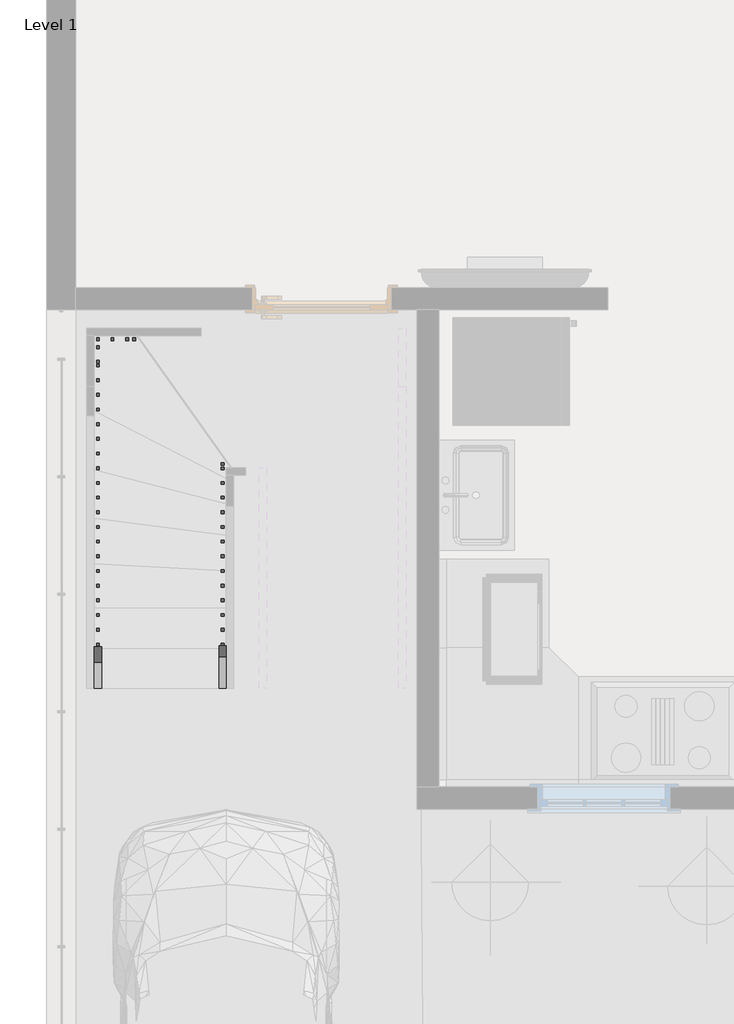
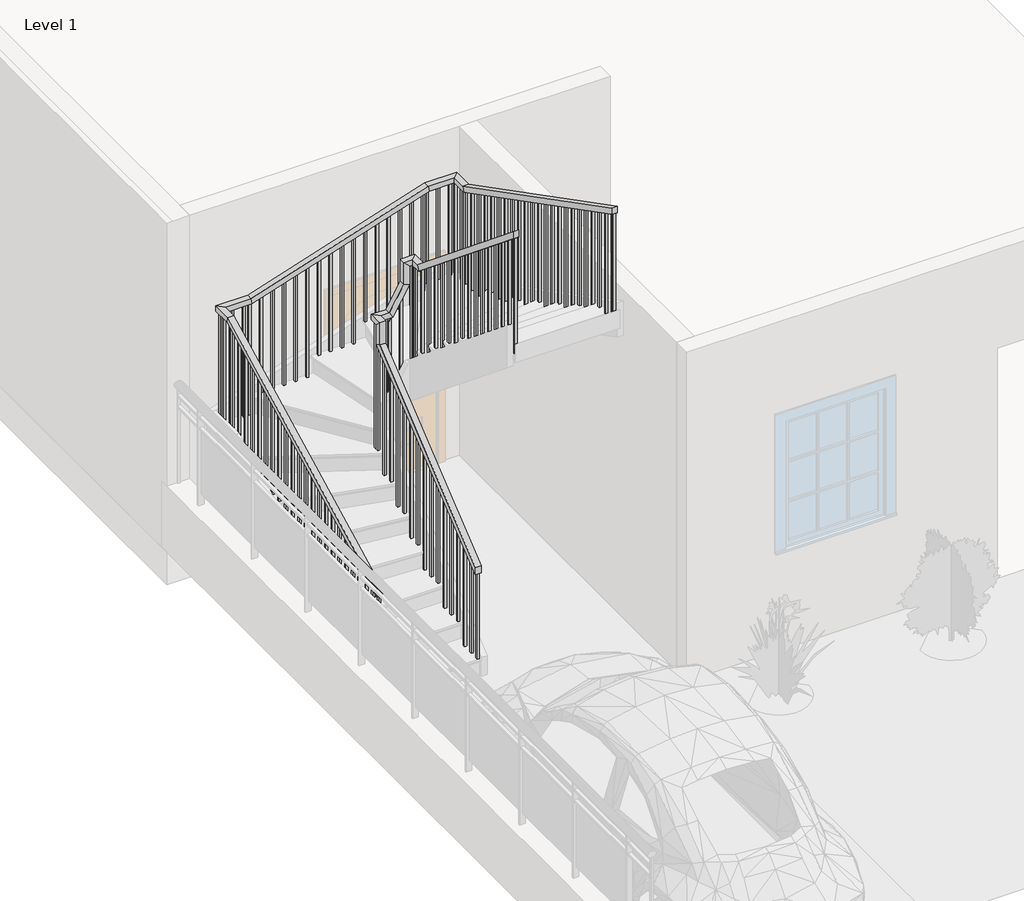
# One storey, part 2 of 3: 2 railings.
"""IFC4 building model written with IfcOpenShell, lengths in millimetres."""

from ifc_helpers import new_model, si_unit, frame, origin, place, context, project, spatial, polyline, outline, extrude, faceted_brep, element, save

model = new_model("IFC4")

# Units and contexts
model_context = context("Model", 3, world=origin())
ifc_project = project(units=[si_unit("LENGTHUNIT", "METRE", prefix="MILLI")], contexts=[model_context])

# Site, building, storey
site = spatial("IfcSite", under=ifc_project)
building = spatial("IfcBuilding", under=site)
storey = spatial("IfcBuildingStorey", under=building, Name="Level 1", Elevation=0.0)

# Railings
placement = place(None, origin())
element("IfcRailing", 1, ObjectType="Handrail - Rectangular", at=placement, inside=storey, context=model_context, shape_type="SolidModel", body=[
    faceted_brep([(-12084.6589543, -3829.6838739, 1025.2529681), (-12084.6589543, -3829.6838739, 959.7067088), (-12033.8589543, -3829.6838739, 959.7067088), (-12033.8589543, -3829.6838739, 1025.2529681), (-12084.6589543, -2378.152182, 2208.7848338), (-12084.6589543, -2327.352182, 2184.659247), (-12033.8589543, -2327.352182, 2184.659247), (-12033.8589543, -2378.152182, 2208.7848338), (-12084.6589543, -2378.152182, 2414.6281882), (-12084.6589543, -2327.352182, 2363.8281882), (-12033.8589543, -2327.352182, 2363.8281882), (-12033.8589543, -2378.152182, 2414.6281882), (-12084.6589543, -2251.152182, 2414.6281882), (-12084.6589543, -2251.152182, 2363.8281882), (-12033.8589543, -2301.952182, 2363.8281882), (-12033.8589543, -2301.952182, 2414.6281882), (-11957.6589543, -2251.152182, 2414.6281882), (-11928.5376204, -2251.152182, 2363.8281882), (-11928.5376204, -2301.952182, 2363.8281882), (-11957.6589543, -2301.952182, 2414.6281882), (-11830.6589543, -2251.152182, 2631.5051451), (-11779.8589543, -2251.152182, 2617.7256424), (-11779.8589543, -2301.952182, 2617.7256424), (-11830.6589543, -2301.952182, 2631.5051451), (-11830.6589543, -2251.152182, 2837.3484995), (-11779.8589543, -2251.152182, 2786.5484995), (-11779.8589543, -2301.952182, 2786.5484995), (-11830.6589543, -2301.952182, 2837.3484995), (-11703.6589543, -2251.152182, 2837.3484995), (-11703.6589543, -2251.152182, 2786.5484995), (-11754.4589543, -2301.952182, 2786.5484995), (-11754.4589543, -2301.952182, 2837.3484995), (-11703.6589543, -2378.152182, 2837.3484995), (-11703.6589543, -2396.2375951, 2786.5484995), (-11754.4589543, -2396.2375951, 2786.5484995), (-11754.4589543, -2378.152182, 2837.3484995), (-11703.6589543, -3829.6838739, 4020.8803652), (-11754.4589543, -3829.6838739, 4020.8803652), (-11754.4589543, -3829.6838739, 3955.3341059), (-11703.6589543, -3829.6838739, 3955.3341059)], [[[0, 1, 2, 3]], [[1, 0, 4, 5]], [[2, 1, 5, 6]], [[3, 2, 6, 7]], [[0, 3, 7, 4]], [[5, 4, 8, 9]], [[6, 5, 9, 10]], [[7, 6, 10, 11]], [[4, 7, 11, 8]], [[9, 8, 12, 13]], [[10, 9, 13, 14]], [[11, 10, 14, 15]], [[8, 11, 15, 12]], [[13, 12, 16, 17]], [[14, 13, 17, 18]], [[15, 14, 18, 19]], [[12, 15, 19, 16]], [[17, 16, 20, 21]], [[18, 17, 21, 22]], [[19, 18, 22, 23]], [[16, 19, 23, 20]], [[21, 20, 24, 25]], [[22, 21, 25, 26]], [[23, 22, 26, 27]], [[20, 23, 27, 24]], [[25, 24, 28, 29]], [[26, 25, 29, 30]], [[27, 26, 30, 31]], [[24, 27, 31, 28]], [[29, 28, 32, 33]], [[30, 29, 33, 34]], [[31, 30, 34, 35]], [[28, 31, 35, 32]], [[36, 37, 38, 39]], [[33, 32, 36, 39]], [[34, 33, 39, 38]], [[35, 34, 38, 37]], [[32, 35, 37, 36]]]),
    extrude(outline(polyline([(-3739.4445384, 3881.7558784), (-3720.3945384, 3866.2231262), (-3720.3945384, 2878.6666667), (-3739.4445384, 2878.6666667), (-3739.4445384, 3881.7558784)])), frame((-11738.5839543, 0.0, 0.0), z_axis=(1.0, 0.0, 0.0), x_axis=(0.0, 1.0, 0.0)), (0.0, 0.0, 1.0), 19.05),
    extrude(outline(polyline([(-3637.8445384, 3798.9145334), (-3618.7945384, 3783.3817813), (-3618.7945384, 2878.6666667), (-3637.8445384, 2878.6666667), (-3637.8445384, 3798.9145334)])), frame((-11738.5839543, 0.0, 0.0), z_axis=(1.0, 0.0, 0.0), x_axis=(0.0, 1.0, 0.0)), (0.0, 0.0, 1.0), 19.05),
    extrude(outline(polyline([(-3536.2445384, 3716.0731885), (-3517.1945384, 3700.5404364), (-3517.1945384, 2709.3333333), (-3536.2445384, 2709.3333333), (-3536.2445384, 3716.0731885)])), frame((-11738.5839543, 0.0, 0.0), z_axis=(1.0, 0.0, 0.0), x_axis=(0.0, 1.0, 0.0)), (0.0, 0.0, 1.0), 19.05),
    extrude(outline(polyline([(-3434.6445384, 3633.2318436), (-3415.5945384, 3617.6990914), (-3415.5945384, 2709.3333333), (-3434.6445384, 2709.3333333), (-3434.6445384, 3633.2318436)])), frame((-11738.5839543, 0.0, 0.0), z_axis=(1.0, 0.0, 0.0), x_axis=(0.0, 1.0, 0.0)), (0.0, 0.0, 1.0), 19.05),
    extrude(outline(polyline([(-3333.0445384, 3550.3904987), (-3313.9945384, 3534.8577465), (-3313.9945384, 2709.3333333), (-3333.0445384, 2709.3333333), (-3333.0445384, 3550.3904987)])), frame((-11738.5839543, 0.0, 0.0), z_axis=(1.0, 0.0, 0.0), x_axis=(0.0, 1.0, 0.0)), (0.0, 0.0, 1.0), 19.05),
    extrude(outline(polyline([(-3231.4445384, 3467.5491538), (-3212.3945384, 3452.0164016), (-3212.3945384, 2540.0), (-3231.4445384, 2540.0), (-3231.4445384, 3467.5491538)])), frame((-11738.5839543, 0.0, 0.0), z_axis=(1.0, 0.0, 0.0), x_axis=(0.0, 1.0, 0.0)), (0.0, 0.0, 1.0), 19.05),
    extrude(outline(polyline([(-3129.8445384, 3384.7078088), (-3110.7945384, 3369.1750567), (-3110.7945384, 2540.0), (-3129.8445384, 2540.0), (-3129.8445384, 3384.7078088)])), frame((-11738.5839543, 0.0, 0.0), z_axis=(1.0, 0.0, 0.0), x_axis=(0.0, 1.0, 0.0)), (0.0, 0.0, 1.0), 19.05),
    extrude(outline(polyline([(-3028.2445384, 3301.8664639), (-3009.1945384, 3286.3337117), (-3009.1945384, 2540.0), (-3028.2445384, 2540.0), (-3028.2445384, 3301.8664639)])), frame((-11738.5839543, 0.0, 0.0), z_axis=(1.0, 0.0, 0.0), x_axis=(0.0, 1.0, 0.0)), (0.0, 0.0, 1.0), 19.05),
    extrude(outline(polyline([(-2926.6445384, 3219.025119), (-2907.5945384, 3203.4923668), (-2907.5945384, 2370.6666667), (-2926.6445384, 2370.6666667), (-2926.6445384, 3219.025119)])), frame((-11738.5839543, 0.0, 0.0), z_axis=(1.0, 0.0, 0.0), x_axis=(0.0, 1.0, 0.0)), (0.0, 0.0, 1.0), 19.05),
    extrude(outline(polyline([(-2825.0445384, 3136.1837741), (-2805.9945384, 3120.6510219), (-2805.9945384, 2370.6666667), (-2825.0445384, 2370.6666667), (-2825.0445384, 3136.1837741)])), frame((-11738.5839543, 0.0, 0.0), z_axis=(1.0, 0.0, 0.0), x_axis=(0.0, 1.0, 0.0)), (0.0, 0.0, 1.0), 19.05),
    extrude(outline(polyline([(-2723.4445384, 3053.3424291), (-2704.3945384, 3037.809677), (-2704.3945384, 2201.3333333), (-2723.4445384, 2201.3333333), (-2723.4445384, 3053.3424291)])), frame((-11738.5839543, 0.0, 0.0), z_axis=(1.0, 0.0, 0.0), x_axis=(0.0, 1.0, 0.0)), (0.0, 0.0, 1.0), 19.05),
    extrude(outline(polyline([(-2621.8445384, 2970.5010842), (-2602.7945384, 2954.9683321), (-2602.7945384, 2201.3333333), (-2621.8445384, 2201.3333333), (-2621.8445384, 2970.5010842)])), frame((-11738.5839543, 0.0, 0.0), z_axis=(1.0, 0.0, 0.0), x_axis=(0.0, 1.0, 0.0)), (0.0, 0.0, 1.0), 19.05),
    extrude(outline(polyline([(-2520.2445384, 2887.6597393), (-2501.1945384, 2872.1269871), (-2501.1945384, 2032.0), (-2520.2445384, 2032.0), (-2520.2445384, 2887.6597393)])), frame((-11738.5839543, 0.0, 0.0), z_axis=(1.0, 0.0, 0.0), x_axis=(0.0, 1.0, 0.0)), (0.0, 0.0, 1.0), 19.05),
    extrude(outline(polyline([(-2418.6445384, 2804.8183944), (-2399.5945384, 2789.2856422), (-2399.5945384, 2032.0), (-2418.6445384, 2032.0), (-2418.6445384, 2804.8183944)])), frame((-11738.5839543, 0.0, 0.0), z_axis=(1.0, 0.0, 0.0), x_axis=(0.0, 1.0, 0.0)), (0.0, 0.0, 1.0), 19.05),
    extrude(outline(polyline([(2529.115018, -11831.7480505), (2496.5834745, -11850.7980505), (1524.0, -11850.7980505), (1524.0, -11831.7480505), (2529.115018, -11831.7480505)])), frame((0.0, -2286.077182, 0.0), z_axis=(0.0, 1.0, 0.0), x_axis=(0.0, 0.0, 1.0)), (0.0, 0.0, 1.0), 19.05),
    extrude(outline(polyline([(2355.6134525, -11933.3480505), (2323.0819089, -11952.3980505), (1524.0, -11952.3980505), (1524.0, -11933.3480505), (2355.6134525, -11933.3480505)])), frame((0.0, -2286.077182, 0.0), z_axis=(0.0, 1.0, 0.0), x_axis=(0.0, 0.0, 1.0)), (0.0, 0.0, 1.0), 19.05),
    extrude(outline(polyline([(-2416.8088739, 2111.7191617), (-2397.7588739, 2127.2519138), (-2397.7588739, 1016.0), (-2416.8088739, 1016.0), (-2416.8088739, 2111.7191617)])), frame((-12068.7839543, 0.0, 0.0), z_axis=(1.0, 0.0, 0.0), x_axis=(0.0, 1.0, 0.0)), (0.0, 0.0, 1.0), 19.05),
    extrude(outline(polyline([(-2518.4088739, 2028.8778167), (-2499.3588739, 2044.4105689), (-2499.3588739, 1016.0), (-2518.4088739, 1016.0), (-2518.4088739, 2028.8778167)])), frame((-12068.7839543, 0.0, 0.0), z_axis=(1.0, 0.0, 0.0), x_axis=(0.0, 1.0, 0.0)), (0.0, 0.0, 1.0), 19.05),
    extrude(outline(polyline([(-2620.0088739, 1946.0364718), (-2600.9588739, 1961.569224), (-2600.9588739, 846.6666667), (-2620.0088739, 846.6666667), (-2620.0088739, 1946.0364718)])), frame((-12068.7839543, 0.0, 0.0), z_axis=(1.0, 0.0, 0.0), x_axis=(0.0, 1.0, 0.0)), (0.0, 0.0, 1.0), 19.05),
    extrude(outline(polyline([(-2721.6088739, 1863.1951269), (-2702.5588739, 1878.7278791), (-2702.5588739, 846.6666667), (-2721.6088739, 846.6666667), (-2721.6088739, 1863.1951269)])), frame((-12068.7839543, 0.0, 0.0), z_axis=(1.0, 0.0, 0.0), x_axis=(0.0, 1.0, 0.0)), (0.0, 0.0, 1.0), 19.05),
    extrude(outline(polyline([(-2823.2088739, 1780.353782), (-2804.1588739, 1795.8865341), (-2804.1588739, 677.3333333), (-2823.2088739, 677.3333333), (-2823.2088739, 1780.353782)])), frame((-12068.7839543, 0.0, 0.0), z_axis=(1.0, 0.0, 0.0), x_axis=(0.0, 1.0, 0.0)), (0.0, 0.0, 1.0), 19.05),
    extrude(outline(polyline([(-2924.8088739, 1697.5124371), (-2905.7588739, 1713.0451892), (-2905.7588739, 677.3333333), (-2924.8088739, 677.3333333), (-2924.8088739, 1697.5124371)])), frame((-12068.7839543, 0.0, 0.0), z_axis=(1.0, 0.0, 0.0), x_axis=(0.0, 1.0, 0.0)), (0.0, 0.0, 1.0), 19.05),
    extrude(outline(polyline([(-3026.4088739, 1614.6710921), (-3007.3588739, 1630.2038443), (-3007.3588739, 508.0), (-3026.4088739, 508.0), (-3026.4088739, 1614.6710921)])), frame((-12068.7839543, 0.0, 0.0), z_axis=(1.0, 0.0, 0.0), x_axis=(0.0, 1.0, 0.0)), (0.0, 0.0, 1.0), 19.05),
    extrude(outline(polyline([(-3128.0088739, 1531.8297472), (-3108.9588739, 1547.3624994), (-3108.9588739, 508.0), (-3128.0088739, 508.0), (-3128.0088739, 1531.8297472)])), frame((-12068.7839543, 0.0, 0.0), z_axis=(1.0, 0.0, 0.0), x_axis=(0.0, 1.0, 0.0)), (0.0, 0.0, 1.0), 19.05),
    extrude(outline(polyline([(-3229.6088739, 1448.9884023), (-3210.5588739, 1464.5211545), (-3210.5588739, 508.0), (-3229.6088739, 508.0), (-3229.6088739, 1448.9884023)])), frame((-12068.7839543, 0.0, 0.0), z_axis=(1.0, 0.0, 0.0), x_axis=(0.0, 1.0, 0.0)), (0.0, 0.0, 1.0), 19.05),
    extrude(outline(polyline([(-3331.2088739, 1366.1470574), (-3312.1588739, 1381.6798095), (-3312.1588739, 338.6666667), (-3331.2088739, 338.6666667), (-3331.2088739, 1366.1470574)])), frame((-12068.7839543, 0.0, 0.0), z_axis=(1.0, 0.0, 0.0), x_axis=(0.0, 1.0, 0.0)), (0.0, 0.0, 1.0), 19.05),
    extrude(outline(polyline([(-3432.8088739, 1283.3057124), (-3413.7588739, 1298.8384646), (-3413.7588739, 338.6666667), (-3432.8088739, 338.6666667), (-3432.8088739, 1283.3057124)])), frame((-12068.7839543, 0.0, 0.0), z_axis=(1.0, 0.0, 0.0), x_axis=(0.0, 1.0, 0.0)), (0.0, 0.0, 1.0), 19.05),
    extrude(outline(polyline([(-3534.4088739, 1200.4643675), (-3515.3588739, 1215.9971197), (-3515.3588739, 338.6666667), (-3534.4088739, 338.6666667), (-3534.4088739, 1200.4643675)])), frame((-12068.7839543, 0.0, 0.0), z_axis=(1.0, 0.0, 0.0), x_axis=(0.0, 1.0, 0.0)), (0.0, 0.0, 1.0), 19.05),
    extrude(outline(polyline([(-3636.0088739, 1117.6230226), (-3616.9588739, 1133.1557748), (-3616.9588739, 169.3333333), (-3636.0088739, 169.3333333), (-3636.0088739, 1117.6230226)])), frame((-12068.7839543, 0.0, 0.0), z_axis=(1.0, 0.0, 0.0), x_axis=(0.0, 1.0, 0.0)), (0.0, 0.0, 1.0), 19.05),
    extrude(outline(polyline([(-3737.6088739, 1034.7816777), (-3718.5588739, 1050.3144298), (-3718.5588739, 169.3333333), (-3737.6088739, 169.3333333), (-3737.6088739, 1034.7816777)])), frame((-12068.7839543, 0.0, 0.0), z_axis=(1.0, 0.0, 0.0), x_axis=(0.0, 1.0, 0.0)), (0.0, 0.0, 1.0), 19.05),
    extrude(outline(polyline([(-11738.5839543, -2297.9945384), (-11719.5339543, -2297.9945384), (-11719.5339543, -2317.0445384), (-11738.5839543, -2317.0445384), (-11738.5839543, -2297.9945384)])), frame((0.0, 0.0, 1862.6666667), z_axis=(0.0, 0.0, 1.0), x_axis=(1.0, 0.0, 0.0)), (0.0, 0.0, 1.0), 923.8818329),
    extrude(outline(polyline([(-11738.5839543, -2286.077182), (-11738.5839543, -2267.027182), (-11719.5339543, -2267.027182), (-11719.5339543, -2286.077182), (-11738.5839543, -2286.077182)])), frame((0.0, 0.0, 1862.6666667), z_axis=(0.0, 0.0, 1.0), x_axis=(1.0, 0.0, 0.0)), (0.0, 0.0, 1.0), 923.8818329),
    extrude(outline(polyline([(-11753.369858, -2286.077182), (-11753.369858, -2267.027182), (-11734.319858, -2267.027182), (-11734.319858, -2286.077182), (-11753.369858, -2286.077182)])), frame((0.0, 0.0, 1693.3333333), z_axis=(0.0, 0.0, 1.0), x_axis=(1.0, 0.0, 0.0)), (0.0, 0.0, 1.0), 1093.2151662),
    extrude(outline(polyline([(-12053.9980505, -2286.077182), (-12053.9980505, -2267.027182), (-12034.9480505, -2267.027182), (-12034.9480505, -2286.077182), (-12053.9980505, -2286.077182)])), frame((0.0, 0.0, 1354.6666667), z_axis=(0.0, 0.0, 1.0), x_axis=(1.0, 0.0, 0.0)), (0.0, 0.0, 1.0), 1009.1615215),
    extrude(outline(polyline([(-12049.7339543, -2286.077182), (-12068.7839543, -2286.077182), (-12068.7839543, -2267.027182), (-12049.7339543, -2267.027182), (-12049.7339543, -2286.077182)])), frame((0.0, 0.0, 1185.3333333), z_axis=(0.0, 0.0, 1.0), x_axis=(1.0, 0.0, 0.0)), (0.0, 0.0, 1.0), 1178.4948549),
    extrude(outline(polyline([(-12049.7339543, -2317.0445384), (-12068.7839543, -2317.0445384), (-12068.7839543, -2297.9945384), (-12049.7339543, -2297.9945384), (-12049.7339543, -2317.0445384)])), frame((0.0, 0.0, 1185.3333333), z_axis=(0.0, 0.0, 1.0), x_axis=(1.0, 0.0, 0.0)), (0.0, 0.0, 1.0), 1178.4948549),
    extrude(outline(polyline([(-3829.6838739, 3955.3341059), (-3810.6338739, 3939.8013537), (-3810.6338739, 2878.6666667), (-3829.6838739, 2878.6666667), (-3829.6838739, 3955.3341059)])), frame((-11738.5839543, 0.0, 0.0), z_axis=(1.0, 0.0, 0.0), x_axis=(0.0, 1.0, 0.0)), (0.0, 0.0, 1.0), 19.05),
    extrude(outline(polyline([(-3829.6838739, 959.7067088), (-3810.6338739, 975.239461), (-3810.6338739, 169.3333333), (-3829.6838739, 169.3333333), (-3829.6838739, 959.7067088)])), frame((-12068.7839543, 0.0, 0.0), z_axis=(1.0, 0.0, 0.0), x_axis=(0.0, 1.0, 0.0)), (0.0, 0.0, 1.0), 19.05),
])
element("IfcRailing", 2, ObjectType="Handrail - Rectangular", at=placement, inside=storey, context=model_context, shape_type="SolidModel", body=[
    faceted_brep([(-12948.2589543, -3829.6838739, 1109.0771751), (-12948.2589543, -3829.6838739, 1051.9280057), (-12897.4589543, -3829.6838739, 1051.9280057), (-12897.4589543, -3829.6838739, 1109.0771751), (-12948.2589543, -1569.7020174, 2273.7644996), (-12948.2589543, -1557.3819661, 2222.9644996), (-12897.4589543, -1557.3819661, 2222.9644996), (-12897.4589543, -1569.7020174, 2273.7644996), (-12948.2589543, -1387.552182, 2273.7644996), (-12948.2589543, -1387.552182, 2222.9644996), (-12897.4589543, -1438.352182, 2222.9644996), (-12897.4589543, -1438.352182, 2273.7644996), (-12671.1050016, -1387.552182, 2273.7644996), (-12663.1544255, -1387.552182, 2222.9644996), (-12663.1544255, -1438.352182, 2222.9644996), (-12671.1050016, -1438.352182, 2273.7644996), (-11117.2129069, -1387.552182, 2772.3688337), (-11109.2623307, -1387.552182, 2721.5688337), (-11109.2623307, -1438.352182, 2721.5688337), (-11117.2129069, -1438.352182, 2772.3688337), (-10840.0589543, -1387.552182, 2772.3688337), (-10840.0589543, -1387.552182, 2721.5688337), (-10890.8589543, -1438.352182, 2721.5688337), (-10890.8589543, -1438.352182, 2772.3688337), (-10840.0589543, -1569.7020174, 2772.3688337), (-10840.0589543, -1582.0220687, 2721.5688337), (-10890.8589543, -1582.0220687, 2721.5688337), (-10890.8589543, -1569.7020174, 2772.3688337), (-10840.0589543, -3829.6838739, 3937.0561582), (-10890.8589543, -3829.6838739, 3937.0561582), (-10890.8589543, -3829.6838739, 3879.9069889), (-10840.0589543, -3829.6838739, 3879.9069889)], [[[0, 1, 2, 3]], [[1, 0, 4, 5]], [[2, 1, 5, 6]], [[3, 2, 6, 7]], [[0, 3, 7, 4]], [[5, 4, 8, 9]], [[6, 5, 9, 10]], [[7, 6, 10, 11]], [[4, 7, 11, 8]], [[9, 8, 12, 13]], [[10, 9, 13, 14]], [[11, 10, 14, 15]], [[8, 11, 15, 12]], [[13, 12, 16, 17]], [[14, 13, 17, 18]], [[15, 14, 18, 19]], [[12, 15, 19, 16]], [[17, 16, 20, 21]], [[18, 17, 21, 22]], [[19, 18, 22, 23]], [[16, 19, 23, 20]], [[21, 20, 24, 25]], [[22, 21, 25, 26]], [[23, 22, 26, 27]], [[20, 23, 27, 24]], [[28, 29, 30, 31]], [[25, 24, 28, 31]], [[26, 25, 31, 30]], [[27, 26, 30, 29]], [[24, 27, 29, 28]]]),
    extrude(outline(polyline([(-3795.3770174, 3862.2268642), (-3795.3770174, 2878.6666667), (-3814.4270174, 2878.6666667), (-3814.4270174, 3872.0443296), (-3795.3770174, 3862.2268642)])), frame((-10874.9839543, 0.0, 0.0), z_axis=(1.0, 0.0, 0.0), x_axis=(0.0, 1.0, 0.0)), (0.0, 0.0, 1.0), 19.05),
    extrude(outline(polyline([(-3693.7770174, 3809.8670491), (-3693.7770174, 2878.6666667), (-3712.8270174, 2878.6666667), (-3712.8270174, 3819.6845145), (-3693.7770174, 3809.8670491)])), frame((-10874.9839543, 0.0, 0.0), z_axis=(1.0, 0.0, 0.0), x_axis=(0.0, 1.0, 0.0)), (0.0, 0.0, 1.0), 19.05),
    extrude(outline(polyline([(-3592.1770174, 3757.507234), (-3592.1770174, 2878.6666667), (-3611.2270174, 2878.6666667), (-3611.2270174, 3767.3246993), (-3592.1770174, 3757.507234)])), frame((-10874.9839543, 0.0, 0.0), z_axis=(1.0, 0.0, 0.0), x_axis=(0.0, 1.0, 0.0)), (0.0, 0.0, 1.0), 19.05),
    extrude(outline(polyline([(-3490.5770174, 3705.1474189), (-3490.5770174, 2709.3333333), (-3509.6270174, 2709.3333333), (-3509.6270174, 3714.9648842), (-3490.5770174, 3705.1474189)])), frame((-10874.9839543, 0.0, 0.0), z_axis=(1.0, 0.0, 0.0), x_axis=(0.0, 1.0, 0.0)), (0.0, 0.0, 1.0), 19.05),
    extrude(outline(polyline([(-3388.9770174, 3652.7876038), (-3388.9770174, 2709.3333333), (-3408.0270174, 2709.3333333), (-3408.0270174, 3662.6050691), (-3388.9770174, 3652.7876038)])), frame((-10874.9839543, 0.0, 0.0), z_axis=(1.0, 0.0, 0.0), x_axis=(0.0, 1.0, 0.0)), (0.0, 0.0, 1.0), 19.05),
    extrude(outline(polyline([(-3287.3770174, 3600.4277887), (-3287.3770174, 2709.3333333), (-3306.4270174, 2709.3333333), (-3306.4270174, 3610.245254), (-3287.3770174, 3600.4277887)])), frame((-10874.9839543, 0.0, 0.0), z_axis=(1.0, 0.0, 0.0), x_axis=(0.0, 1.0, 0.0)), (0.0, 0.0, 1.0), 19.05),
    extrude(outline(polyline([(-3185.7770174, 3548.0679735), (-3185.7770174, 2540.0), (-3204.8270174, 2540.0), (-3204.8270174, 3557.8854389), (-3185.7770174, 3548.0679735)])), frame((-10874.9839543, 0.0, 0.0), z_axis=(1.0, 0.0, 0.0), x_axis=(0.0, 1.0, 0.0)), (0.0, 0.0, 1.0), 19.05),
    extrude(outline(polyline([(-3084.1770174, 3495.7081584), (-3084.1770174, 2540.0), (-3103.2270174, 2540.0), (-3103.2270174, 3505.5256238), (-3084.1770174, 3495.7081584)])), frame((-10874.9839543, 0.0, 0.0), z_axis=(1.0, 0.0, 0.0), x_axis=(0.0, 1.0, 0.0)), (0.0, 0.0, 1.0), 19.05),
    extrude(outline(polyline([(-2982.5770174, 3443.3483433), (-2982.5770174, 2540.0), (-3001.6270174, 2540.0), (-3001.6270174, 3453.1658086), (-2982.5770174, 3443.3483433)])), frame((-10874.9839543, 0.0, 0.0), z_axis=(1.0, 0.0, 0.0), x_axis=(0.0, 1.0, 0.0)), (0.0, 0.0, 1.0), 19.05),
    extrude(outline(polyline([(-2880.9770174, 3390.9885282), (-2880.9770174, 2370.6666667), (-2900.0270174, 2370.6666667), (-2900.0270174, 3400.8059935), (-2880.9770174, 3390.9885282)])), frame((-10874.9839543, 0.0, 0.0), z_axis=(1.0, 0.0, 0.0), x_axis=(0.0, 1.0, 0.0)), (0.0, 0.0, 1.0), 19.05),
    extrude(outline(polyline([(-2779.3770174, 3338.6287131), (-2779.3770174, 2370.6666667), (-2798.4270174, 2370.6666667), (-2798.4270174, 3348.4461784), (-2779.3770174, 3338.6287131)])), frame((-10874.9839543, 0.0, 0.0), z_axis=(1.0, 0.0, 0.0), x_axis=(0.0, 1.0, 0.0)), (0.0, 0.0, 1.0), 19.05),
    extrude(outline(polyline([(-2677.7770174, 3286.268898), (-2677.7770174, 2370.6666667), (-2696.8270174, 2370.6666667), (-2696.8270174, 3296.0863633), (-2677.7770174, 3286.268898)])), frame((-10874.9839543, 0.0, 0.0), z_axis=(1.0, 0.0, 0.0), x_axis=(0.0, 1.0, 0.0)), (0.0, 0.0, 1.0), 19.05),
    extrude(outline(polyline([(-2576.1770174, 3233.9090828), (-2576.1770174, 2201.3333333), (-2595.2270174, 2201.3333333), (-2595.2270174, 3243.7265482), (-2576.1770174, 3233.9090828)])), frame((-10874.9839543, 0.0, 0.0), z_axis=(1.0, 0.0, 0.0), x_axis=(0.0, 1.0, 0.0)), (0.0, 0.0, 1.0), 19.05),
    extrude(outline(polyline([(-2474.5770174, 3181.5492677), (-2474.5770174, 2201.3333333), (-2493.6270174, 2201.3333333), (-2493.6270174, 3191.3667331), (-2474.5770174, 3181.5492677)])), frame((-10874.9839543, 0.0, 0.0), z_axis=(1.0, 0.0, 0.0), x_axis=(0.0, 1.0, 0.0)), (0.0, 0.0, 1.0), 19.05),
    extrude(outline(polyline([(-2372.9770174, 3129.1894526), (-2372.9770174, 2201.3333333), (-2392.0270174, 2201.3333333), (-2392.0270174, 3139.0069179), (-2372.9770174, 3129.1894526)])), frame((-10874.9839543, 0.0, 0.0), z_axis=(1.0, 0.0, 0.0), x_axis=(0.0, 1.0, 0.0)), (0.0, 0.0, 1.0), 19.05),
    extrude(outline(polyline([(-2271.3770174, 3076.8296375), (-2271.3770174, 2032.0), (-2290.4270174, 2032.0), (-2290.4270174, 3086.6471028), (-2271.3770174, 3076.8296375)])), frame((-10874.9839543, 0.0, 0.0), z_axis=(1.0, 0.0, 0.0), x_axis=(0.0, 1.0, 0.0)), (0.0, 0.0, 1.0), 19.05),
    extrude(outline(polyline([(-2169.7770174, 3024.4698224), (-2169.7770174, 2032.0), (-2188.8270174, 2032.0), (-2188.8270174, 3034.2872877), (-2169.7770174, 3024.4698224)])), frame((-10874.9839543, 0.0, 0.0), z_axis=(1.0, 0.0, 0.0), x_axis=(0.0, 1.0, 0.0)), (0.0, 0.0, 1.0), 19.05),
    extrude(outline(polyline([(-2068.1770174, 2972.1100073), (-2068.1770174, 2032.0), (-2087.2270174, 2032.0), (-2087.2270174, 2981.9274726), (-2068.1770174, 2972.1100073)])), frame((-10874.9839543, 0.0, 0.0), z_axis=(1.0, 0.0, 0.0), x_axis=(0.0, 1.0, 0.0)), (0.0, 0.0, 1.0), 19.05),
    extrude(outline(polyline([(-1966.5770174, 2919.7501921), (-1966.5770174, 2032.0), (-1985.6270174, 2032.0), (-1985.6270174, 2929.5676575), (-1966.5770174, 2919.7501921)])), frame((-10874.9839543, 0.0, 0.0), z_axis=(1.0, 0.0, 0.0), x_axis=(0.0, 1.0, 0.0)), (0.0, 0.0, 1.0), 19.05),
    extrude(outline(polyline([(-1864.9770174, 2867.390377), (-1864.9770174, 1862.6666667), (-1884.0270174, 1862.6666667), (-1884.0270174, 2877.2078424), (-1864.9770174, 2867.390377)])), frame((-10874.9839543, 0.0, 0.0), z_axis=(1.0, 0.0, 0.0), x_axis=(0.0, 1.0, 0.0)), (0.0, 0.0, 1.0), 19.05),
    extrude(outline(polyline([(-1763.3770174, 2815.0305619), (-1763.3770174, 1862.6666667), (-1782.4270174, 1862.6666667), (-1782.4270174, 2824.8480272), (-1763.3770174, 2815.0305619)])), frame((-10874.9839543, 0.0, 0.0), z_axis=(1.0, 0.0, 0.0), x_axis=(0.0, 1.0, 0.0)), (0.0, 0.0, 1.0), 19.05),
    extrude(outline(polyline([(-1661.7770174, 2762.6707468), (-1661.7770174, 1862.6666667), (-1680.8270174, 1862.6666667), (-1680.8270174, 2772.4882121), (-1661.7770174, 2762.6707468)])), frame((-10874.9839543, 0.0, 0.0), z_axis=(1.0, 0.0, 0.0), x_axis=(0.0, 1.0, 0.0)), (0.0, 0.0, 1.0), 19.05),
    extrude(outline(polyline([(-10855.9339543, -1505.027182), (-10855.9339543, -1524.077182), (-10874.9839543, -1524.077182), (-10874.9839543, -1505.027182), (-10855.9339543, -1505.027182)])), frame((0.0, 0.0, 1862.6666667), z_axis=(0.0, 0.0, 1.0), x_axis=(1.0, 0.0, 0.0)), (0.0, 0.0, 1.0), 858.902167),
    extrude(outline(polyline([(-10923.5379069, -1403.427182), (-10904.4879069, -1403.427182), (-10904.4879069, -1422.477182), (-10923.5379069, -1422.477182), (-10923.5379069, -1403.427182)])), frame((0.0, 0.0, 1862.6666667), z_axis=(0.0, 0.0, 1.0), x_axis=(1.0, 0.0, 0.0)), (0.0, 0.0, 1.0), 858.902167),
    extrude(outline(polyline([(-11025.1379069, -1403.427182), (-11006.0879069, -1403.427182), (-11006.0879069, -1422.477182), (-11025.1379069, -1422.477182), (-11025.1379069, -1403.427182)])), frame((0.0, 0.0, 1862.6666667), z_axis=(0.0, 0.0, 1.0), x_axis=(1.0, 0.0, 0.0)), (0.0, 0.0, 1.0), 858.902167),
    extrude(outline(polyline([(2706.3697564, -11156.6300016), (1693.3333333, -11156.6300016), (1693.3333333, -11137.5800016), (2712.4824155, -11137.5800016), (2706.3697564, -11156.6300016)])), frame((0.0, -1422.477182, 0.0), z_axis=(0.0, 1.0, 0.0), x_axis=(0.0, 0.0, 1.0)), (0.0, 0.0, 1.0), 19.05),
    extrude(outline(polyline([(2673.7689082, -11258.2300016), (1693.3333333, -11258.2300016), (1693.3333333, -11239.1800016), (2679.8815673, -11239.1800016), (2673.7689082, -11258.2300016)])), frame((0.0, -1422.477182, 0.0), z_axis=(0.0, 1.0, 0.0), x_axis=(0.0, 0.0, 1.0)), (0.0, 0.0, 1.0), 19.05),
    extrude(outline(polyline([(2641.16806, -11359.8300016), (1693.3333333, -11359.8300016), (1693.3333333, -11340.7800016), (2647.280719, -11340.7800016), (2641.16806, -11359.8300016)])), frame((0.0, -1422.477182, 0.0), z_axis=(0.0, 1.0, 0.0), x_axis=(0.0, 0.0, 1.0)), (0.0, 0.0, 1.0), 19.05),
    extrude(outline(polyline([(2608.5672118, -11461.4300016), (1693.3333333, -11461.4300016), (1693.3333333, -11442.3800016), (2614.6798708, -11442.3800016), (2608.5672118, -11461.4300016)])), frame((0.0, -1422.477182, 0.0), z_axis=(0.0, 1.0, 0.0), x_axis=(0.0, 0.0, 1.0)), (0.0, 0.0, 1.0), 19.05),
    extrude(outline(polyline([(2575.9663635, -11563.0300016), (1693.3333333, -11563.0300016), (1693.3333333, -11543.9800016), (2582.0790226, -11543.9800016), (2575.9663635, -11563.0300016)])), frame((0.0, -1422.477182, 0.0), z_axis=(0.0, 1.0, 0.0), x_axis=(0.0, 0.0, 1.0)), (0.0, 0.0, 1.0), 19.05),
    extrude(outline(polyline([(2543.3655153, -11664.6300016), (1693.3333333, -11664.6300016), (1693.3333333, -11645.5800016), (2549.4781744, -11645.5800016), (2543.3655153, -11664.6300016)])), frame((0.0, -1422.477182, 0.0), z_axis=(0.0, 1.0, 0.0), x_axis=(0.0, 0.0, 1.0)), (0.0, 0.0, 1.0), 19.05),
    extrude(outline(polyline([(2510.7646671, -11766.2300016), (1524.0, -11766.2300016), (1524.0, -11747.1800016), (2516.8773261, -11747.1800016), (2510.7646671, -11766.2300016)])), frame((0.0, -1422.477182, 0.0), z_axis=(0.0, 1.0, 0.0), x_axis=(0.0, 0.0, 1.0)), (0.0, 0.0, 1.0), 19.05),
    extrude(outline(polyline([(2478.1638189, -11867.8300016), (1524.0, -11867.8300016), (1524.0, -11848.7800016), (2484.2764779, -11848.7800016), (2478.1638189, -11867.8300016)])), frame((0.0, -1422.477182, 0.0), z_axis=(0.0, 1.0, 0.0), x_axis=(0.0, 0.0, 1.0)), (0.0, 0.0, 1.0), 19.05),
    extrude(outline(polyline([(2445.5629706, -11969.4300016), (1524.0, -11969.4300016), (1524.0, -11950.3800016), (2451.6756297, -11950.3800016), (2445.5629706, -11969.4300016)])), frame((0.0, -1422.477182, 0.0), z_axis=(0.0, 1.0, 0.0), x_axis=(0.0, 0.0, 1.0)), (0.0, 0.0, 1.0), 19.05),
    extrude(outline(polyline([(2412.9621224, -12071.0300016), (1524.0, -12071.0300016), (1524.0, -12051.9800016), (2419.0747814, -12051.9800016), (2412.9621224, -12071.0300016)])), frame((0.0, -1422.477182, 0.0), z_axis=(0.0, 1.0, 0.0), x_axis=(0.0, 0.0, 1.0)), (0.0, 0.0, 1.0), 19.05),
    extrude(outline(polyline([(2380.3612742, -12172.6300016), (1354.6666667, -12172.6300016), (1354.6666667, -12153.5800016), (2386.4739332, -12153.5800016), (2380.3612742, -12172.6300016)])), frame((0.0, -1422.477182, 0.0), z_axis=(0.0, 1.0, 0.0), x_axis=(0.0, 0.0, 1.0)), (0.0, 0.0, 1.0), 19.05),
    extrude(outline(polyline([(2347.7604259, -12274.2300016), (1354.6666667, -12274.2300016), (1354.6666667, -12255.1800016), (2353.873085, -12255.1800016), (2347.7604259, -12274.2300016)])), frame((0.0, -1422.477182, 0.0), z_axis=(0.0, 1.0, 0.0), x_axis=(0.0, 0.0, 1.0)), (0.0, 0.0, 1.0), 19.05),
    extrude(outline(polyline([(2315.1595777, -12375.8300016), (1354.6666667, -12375.8300016), (1354.6666667, -12356.7800016), (2321.2722368, -12356.7800016), (2315.1595777, -12375.8300016)])), frame((0.0, -1422.477182, 0.0), z_axis=(0.0, 1.0, 0.0), x_axis=(0.0, 0.0, 1.0)), (0.0, 0.0, 1.0), 19.05),
    extrude(outline(polyline([(2282.5587295, -12477.4300016), (1354.6666667, -12477.4300016), (1354.6666667, -12458.3800016), (2288.6713885, -12458.3800016), (2282.5587295, -12477.4300016)])), frame((0.0, -1422.477182, 0.0), z_axis=(0.0, 1.0, 0.0), x_axis=(0.0, 0.0, 1.0)), (0.0, 0.0, 1.0), 19.05),
    extrude(outline(polyline([(2249.9578813, -12579.0300016), (1354.6666667, -12579.0300016), (1354.6666667, -12559.9800016), (2256.0705403, -12559.9800016), (2249.9578813, -12579.0300016)])), frame((0.0, -1422.477182, 0.0), z_axis=(0.0, 1.0, 0.0), x_axis=(0.0, 0.0, 1.0)), (0.0, 0.0, 1.0), 19.05),
    extrude(outline(polyline([(-12729.1839543, -1403.427182), (-12710.1339543, -1403.427182), (-12710.1339543, -1422.477182), (-12729.1839543, -1422.477182), (-12729.1839543, -1403.427182)])), frame((0.0, 0.0, 1185.3333333), z_axis=(0.0, 0.0, 1.0), x_axis=(1.0, 0.0, 0.0)), (0.0, 0.0, 1.0), 1037.6311663),
    extrude(outline(polyline([(-12830.7839543, -1403.427182), (-12811.7339543, -1403.427182), (-12811.7339543, -1422.477182), (-12830.7839543, -1422.477182), (-12830.7839543, -1403.427182)])), frame((0.0, 0.0, 1185.3333333), z_axis=(0.0, 0.0, 1.0), x_axis=(1.0, 0.0, 0.0)), (0.0, 0.0, 1.0), 1037.6311663),
    extrude(outline(polyline([(-12932.3839543, -1477.6270174), (-12932.3839543, -1458.5770174), (-12913.3339543, -1458.5770174), (-12913.3339543, -1477.6270174), (-12932.3839543, -1477.6270174)])), frame((0.0, 0.0, 1185.3333333), z_axis=(0.0, 0.0, 1.0), x_axis=(1.0, 0.0, 0.0)), (0.0, 0.0, 1.0), 1037.6311663),
    extrude(outline(polyline([(-1584.9588739, 2208.752671), (-1584.9588739, 1185.3333333), (-1604.0088739, 1185.3333333), (-1604.0088739, 2198.9352056), (-1584.9588739, 2208.752671)])), frame((-12932.3839543, 0.0, 0.0), z_axis=(1.0, 0.0, 0.0), x_axis=(0.0, 1.0, 0.0)), (0.0, 0.0, 1.0), 19.05),
    extrude(outline(polyline([(-1686.5588739, 2156.3928558), (-1686.5588739, 1185.3333333), (-1705.6088739, 1185.3333333), (-1705.6088739, 2146.5753905), (-1686.5588739, 2156.3928558)])), frame((-12932.3839543, 0.0, 0.0), z_axis=(1.0, 0.0, 0.0), x_axis=(0.0, 1.0, 0.0)), (0.0, 0.0, 1.0), 19.05),
    extrude(outline(polyline([(-1788.1588739, 2104.0330407), (-1788.1588739, 1185.3333333), (-1807.2088739, 1185.3333333), (-1807.2088739, 2094.2155754), (-1788.1588739, 2104.0330407)])), frame((-12932.3839543, 0.0, 0.0), z_axis=(1.0, 0.0, 0.0), x_axis=(0.0, 1.0, 0.0)), (0.0, 0.0, 1.0), 19.05),
    extrude(outline(polyline([(-1889.7588739, 2051.6732256), (-1889.7588739, 1185.3333333), (-1908.8088739, 1185.3333333), (-1908.8088739, 2041.8557603), (-1889.7588739, 2051.6732256)])), frame((-12932.3839543, 0.0, 0.0), z_axis=(1.0, 0.0, 0.0), x_axis=(0.0, 1.0, 0.0)), (0.0, 0.0, 1.0), 19.05),
    extrude(outline(polyline([(-1991.3588739, 1999.3134105), (-1991.3588739, 1016.0), (-2010.4088739, 1016.0), (-2010.4088739, 1989.4959452), (-1991.3588739, 1999.3134105)])), frame((-12932.3839543, 0.0, 0.0), z_axis=(1.0, 0.0, 0.0), x_axis=(0.0, 1.0, 0.0)), (0.0, 0.0, 1.0), 19.05),
    extrude(outline(polyline([(-2092.9588739, 1946.9535954), (-2092.9588739, 1016.0), (-2112.0088739, 1016.0), (-2112.0088739, 1937.13613), (-2092.9588739, 1946.9535954)])), frame((-12932.3839543, 0.0, 0.0), z_axis=(1.0, 0.0, 0.0), x_axis=(0.0, 1.0, 0.0)), (0.0, 0.0, 1.0), 19.05),
    extrude(outline(polyline([(-2194.5588739, 1894.5937803), (-2194.5588739, 1016.0), (-2213.6088739, 1016.0), (-2213.6088739, 1884.7763149), (-2194.5588739, 1894.5937803)])), frame((-12932.3839543, 0.0, 0.0), z_axis=(1.0, 0.0, 0.0), x_axis=(0.0, 1.0, 0.0)), (0.0, 0.0, 1.0), 19.05),
    extrude(outline(polyline([(-2296.1588739, 1842.2339651), (-2296.1588739, 1016.0), (-2315.2088739, 1016.0), (-2315.2088739, 1832.4164998), (-2296.1588739, 1842.2339651)])), frame((-12932.3839543, 0.0, 0.0), z_axis=(1.0, 0.0, 0.0), x_axis=(0.0, 1.0, 0.0)), (0.0, 0.0, 1.0), 19.05),
    extrude(outline(polyline([(-2397.7588739, 1789.87415), (-2397.7588739, 846.6666667), (-2416.8088739, 846.6666667), (-2416.8088739, 1780.0566847), (-2397.7588739, 1789.87415)])), frame((-12932.3839543, 0.0, 0.0), z_axis=(1.0, 0.0, 0.0), x_axis=(0.0, 1.0, 0.0)), (0.0, 0.0, 1.0), 19.05),
    extrude(outline(polyline([(-2499.3588739, 1737.5143349), (-2499.3588739, 846.6666667), (-2518.4088739, 846.6666667), (-2518.4088739, 1727.6968696), (-2499.3588739, 1737.5143349)])), frame((-12932.3839543, 0.0, 0.0), z_axis=(1.0, 0.0, 0.0), x_axis=(0.0, 1.0, 0.0)), (0.0, 0.0, 1.0), 19.05),
    extrude(outline(polyline([(-2600.9588739, 1685.1545198), (-2600.9588739, 846.6666667), (-2620.0088739, 846.6666667), (-2620.0088739, 1675.3370545), (-2600.9588739, 1685.1545198)])), frame((-12932.3839543, 0.0, 0.0), z_axis=(1.0, 0.0, 0.0), x_axis=(0.0, 1.0, 0.0)), (0.0, 0.0, 1.0), 19.05),
    extrude(outline(polyline([(-2702.5588739, 1632.7947047), (-2702.5588739, 677.3333333), (-2721.6088739, 677.3333333), (-2721.6088739, 1622.9772393), (-2702.5588739, 1632.7947047)])), frame((-12932.3839543, 0.0, 0.0), z_axis=(1.0, 0.0, 0.0), x_axis=(0.0, 1.0, 0.0)), (0.0, 0.0, 1.0), 19.05),
    extrude(outline(polyline([(-2804.1588739, 1580.4348896), (-2804.1588739, 677.3333333), (-2823.2088739, 677.3333333), (-2823.2088739, 1570.6174242), (-2804.1588739, 1580.4348896)])), frame((-12932.3839543, 0.0, 0.0), z_axis=(1.0, 0.0, 0.0), x_axis=(0.0, 1.0, 0.0)), (0.0, 0.0, 1.0), 19.05),
    extrude(outline(polyline([(-2905.7588739, 1528.0750744), (-2905.7588739, 677.3333333), (-2924.8088739, 677.3333333), (-2924.8088739, 1518.2576091), (-2905.7588739, 1528.0750744)])), frame((-12932.3839543, 0.0, 0.0), z_axis=(1.0, 0.0, 0.0), x_axis=(0.0, 1.0, 0.0)), (0.0, 0.0, 1.0), 19.05),
    extrude(outline(polyline([(-3007.3588739, 1475.7152593), (-3007.3588739, 508.0), (-3026.4088739, 508.0), (-3026.4088739, 1465.897794), (-3007.3588739, 1475.7152593)])), frame((-12932.3839543, 0.0, 0.0), z_axis=(1.0, 0.0, 0.0), x_axis=(0.0, 1.0, 0.0)), (0.0, 0.0, 1.0), 19.05),
    extrude(outline(polyline([(-3108.9588739, 1423.3554442), (-3108.9588739, 508.0), (-3128.0088739, 508.0), (-3128.0088739, 1413.5379789), (-3108.9588739, 1423.3554442)])), frame((-12932.3839543, 0.0, 0.0), z_axis=(1.0, 0.0, 0.0), x_axis=(0.0, 1.0, 0.0)), (0.0, 0.0, 1.0), 19.05),
    extrude(outline(polyline([(-3210.5588739, 1370.9956291), (-3210.5588739, 508.0), (-3229.6088739, 508.0), (-3229.6088739, 1361.1781638), (-3210.5588739, 1370.9956291)])), frame((-12932.3839543, 0.0, 0.0), z_axis=(1.0, 0.0, 0.0), x_axis=(0.0, 1.0, 0.0)), (0.0, 0.0, 1.0), 19.05),
    extrude(outline(polyline([(-3312.1588739, 1318.635814), (-3312.1588739, 338.6666667), (-3331.2088739, 338.6666667), (-3331.2088739, 1308.8183486), (-3312.1588739, 1318.635814)])), frame((-12932.3839543, 0.0, 0.0), z_axis=(1.0, 0.0, 0.0), x_axis=(0.0, 1.0, 0.0)), (0.0, 0.0, 1.0), 19.05),
    extrude(outline(polyline([(-3413.7588739, 1266.2759989), (-3413.7588739, 338.6666667), (-3432.8088739, 338.6666667), (-3432.8088739, 1256.4585335), (-3413.7588739, 1266.2759989)])), frame((-12932.3839543, 0.0, 0.0), z_axis=(1.0, 0.0, 0.0), x_axis=(0.0, 1.0, 0.0)), (0.0, 0.0, 1.0), 19.05),
    extrude(outline(polyline([(-3515.3588739, 1213.9161837), (-3515.3588739, 338.6666667), (-3534.4088739, 338.6666667), (-3534.4088739, 1204.0987184), (-3515.3588739, 1213.9161837)])), frame((-12932.3839543, 0.0, 0.0), z_axis=(1.0, 0.0, 0.0), x_axis=(0.0, 1.0, 0.0)), (0.0, 0.0, 1.0), 19.05),
    extrude(outline(polyline([(-3616.9588739, 1161.5563686), (-3616.9588739, 169.3333333), (-3636.0088739, 169.3333333), (-3636.0088739, 1151.7389033), (-3616.9588739, 1161.5563686)])), frame((-12932.3839543, 0.0, 0.0), z_axis=(1.0, 0.0, 0.0), x_axis=(0.0, 1.0, 0.0)), (0.0, 0.0, 1.0), 19.05),
    extrude(outline(polyline([(-3718.5588739, 1109.1965535), (-3718.5588739, 169.3333333), (-3737.6088739, 169.3333333), (-3737.6088739, 1099.3790882), (-3718.5588739, 1109.1965535)])), frame((-12932.3839543, 0.0, 0.0), z_axis=(1.0, 0.0, 0.0), x_axis=(0.0, 1.0, 0.0)), (0.0, 0.0, 1.0), 19.05),
    extrude(outline(polyline([(-10855.9339543, -1560.1770174), (-10855.9339543, -1579.2270174), (-10874.9839543, -1579.2270174), (-10874.9839543, -1560.1770174), (-10855.9339543, -1560.1770174)])), frame((0.0, 0.0, 1862.6666667), z_axis=(0.0, 0.0, 1.0), x_axis=(1.0, 0.0, 0.0)), (0.0, 0.0, 1.0), 858.902167),
    extrude(outline(polyline([(-10874.9839543, -1403.427182), (-10855.9339543, -1403.427182), (-10855.9339543, -1422.477182), (-10874.9839543, -1422.477182), (-10874.9839543, -1403.427182)])), frame((0.0, 0.0, 1862.6666667), z_axis=(0.0, 0.0, 1.0), x_axis=(1.0, 0.0, 0.0)), (0.0, 0.0, 1.0), 858.902167),
    extrude(outline(polyline([(2715.9613671, -11126.7379069), (1862.6666667, -11126.7379069), (1862.6666667, -11107.6879069), (2722.0740262, -11107.6879069), (2715.9613671, -11126.7379069)])), frame((0.0, -1422.477182, 0.0), z_axis=(0.0, 1.0, 0.0), x_axis=(0.0, 0.0, 1.0)), (0.0, 0.0, 1.0), 19.05),
    extrude(outline(polyline([(-12680.6300016, -1403.427182), (-12661.5800016, -1403.427182), (-12661.5800016, -1422.477182), (-12680.6300016, -1422.477182), (-12680.6300016, -1403.427182)])), frame((0.0, 0.0, 1185.3333333), z_axis=(0.0, 0.0, 1.0), x_axis=(1.0, 0.0, 0.0)), (0.0, 0.0, 1.0), 1037.6311663),
    extrude(outline(polyline([(-12932.3839543, -1422.477182), (-12932.3839543, -1403.427182), (-12913.3339543, -1403.427182), (-12913.3339543, -1422.477182), (-12932.3839543, -1422.477182)])), frame((0.0, 0.0, 1185.3333333), z_axis=(0.0, 0.0, 1.0), x_axis=(1.0, 0.0, 0.0)), (0.0, 0.0, 1.0), 1037.6311663),
    extrude(outline(polyline([(-1560.1770174, 2221.5240629), (-1560.1770174, 1185.3333333), (-1579.2270174, 1185.3333333), (-1579.2270174, 2211.7065976), (-1560.1770174, 2221.5240629)])), frame((-12932.3839543, 0.0, 0.0), z_axis=(1.0, 0.0, 0.0), x_axis=(0.0, 1.0, 0.0)), (0.0, 0.0, 1.0), 19.05),
    extrude(outline(polyline([(-3810.6338739, 3870.0895235), (-3810.6338739, 2878.6666667), (-3829.6838739, 2878.6666667), (-3829.6838739, 3879.9069889), (-3810.6338739, 3870.0895235)])), frame((-10874.9839543, 0.0, 0.0), z_axis=(1.0, 0.0, 0.0), x_axis=(0.0, 1.0, 0.0)), (0.0, 0.0, 1.0), 19.05),
    extrude(outline(polyline([(-3810.6338739, 1061.7454711), (-3810.6338739, 169.3333333), (-3829.6838739, 169.3333333), (-3829.6838739, 1051.9280057), (-3810.6338739, 1061.7454711)])), frame((-12932.3839543, 0.0, 0.0), z_axis=(1.0, 0.0, 0.0), x_axis=(0.0, 1.0, 0.0)), (0.0, 0.0, 1.0), 19.05),
])

save(model, "model.ifc")

# Revit data of these elements
# Type "Handrail - Rectangular"
#   Assembly Code = "C2010400"
#   built-in parameter 1008612 = 0.0416667 (stored number, unit not read)
#   built-in parameter 1008611 = 0.0416667 (stored number, unit not read)
#   built-in parameter 1008609 = 0.333333 (stored number, unit not read)
#   built-in parameter 1008604 = 0.166667 (stored number, unit not read)
#   built-in parameter 1008603 = 0.166667 (stored number, unit not read)
#   Railing Height = 3' - 0"
#   built-in parameter 1008630 = 2
#   built-in parameter 1008610 = 2
#   built-in parameter 1008618 = Baluster - Square : 3/4"
# Elements 1, 2 (IfcRailing, "Handrail - Rectangular")
#   Phase Created = New Construction
